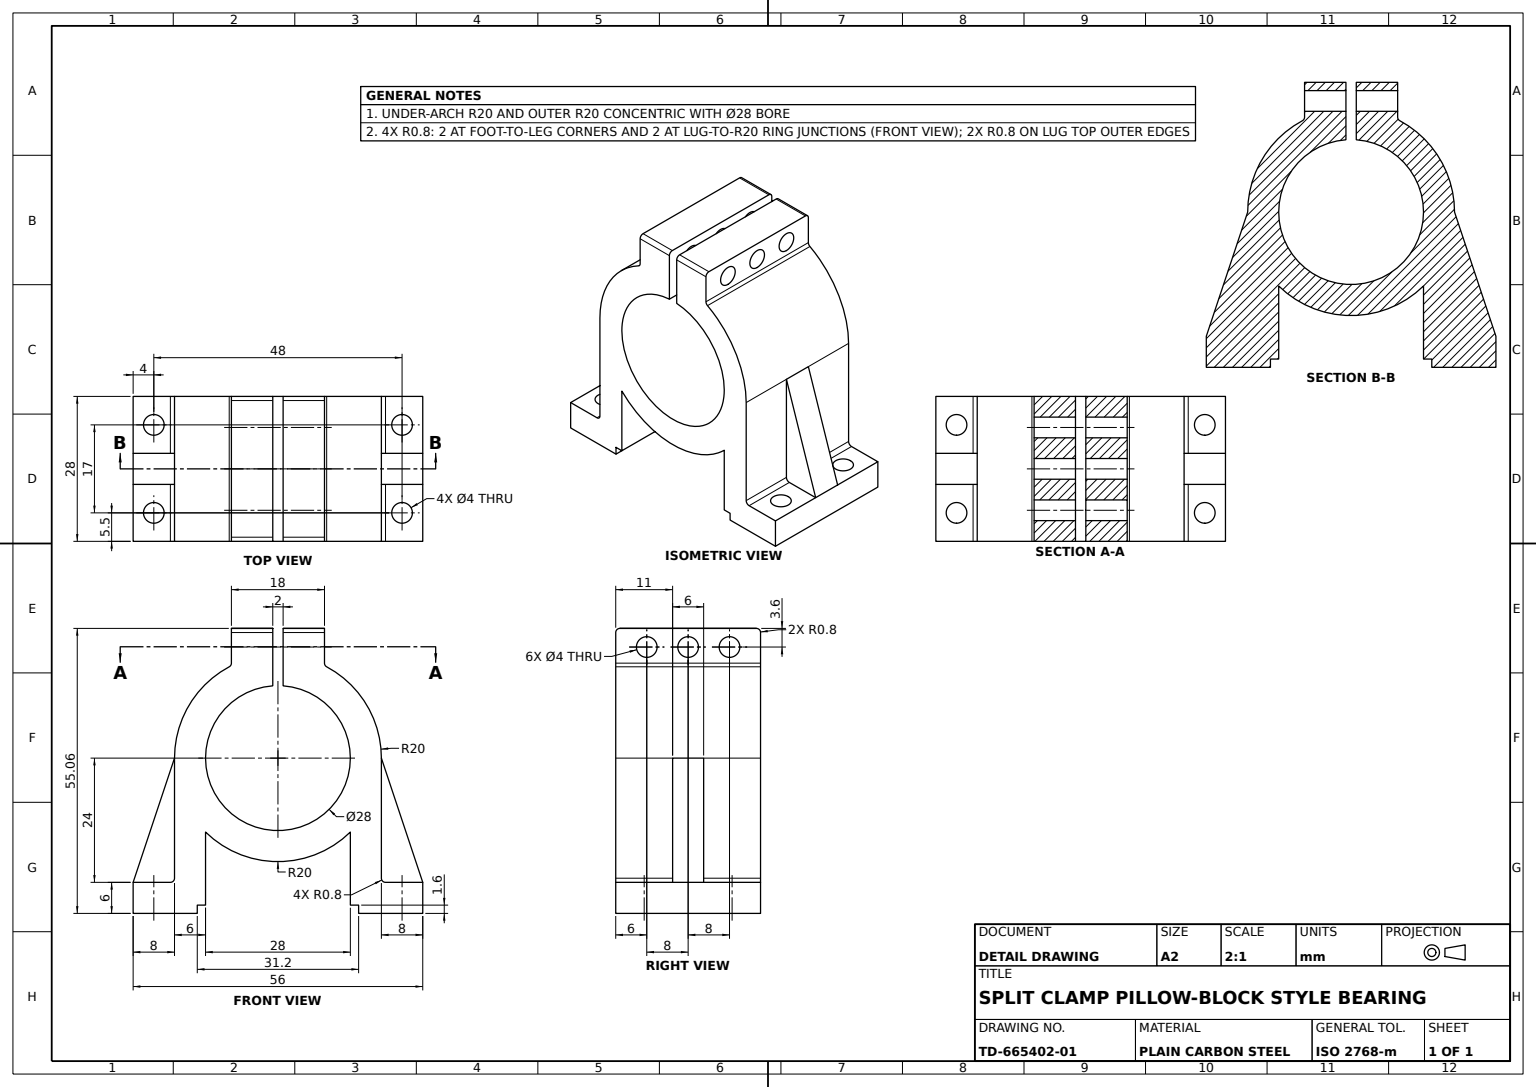
SolidWorks part; units mm, degrees
material "Plain Carbon Steel"
ref_plane "Front Plane" through (0, 0, 0) normal (0, 0, 1) x (1, 0, 0)
ref_plane "Top Plane" through (0, 0, 0) normal (0, 1, 0) x (1, 0, 0)
ref_plane "Right Plane" through (0, 0, 0) normal (1, 0, 0) x (0, 0, -1)
sketch "Omega Profile Sketch" plane through (0, 0, 0) normal (0, 0, 1) x (1, 0, 0)
  line L0 (-20, 0) -> (-20, -24)
  line L1 (-20, -24) -> (-28, -24)
  line L2 (-28, -24) -> (-28, -30)
  line L3 (-28, -30) -> (-15.6, -30)
  line L4 (-14, -28.4) -> (-14, -14.2829)
  line L5 (-14, -28.4) -> (-15.6, -28.4)
  line L6 (-15.6, -28.4) -> (-15.6, -30)
  line L7 (20, 0) -> (20, -24)
  line L8 (20, -24) -> (28, -24)
  line L9 (28, -24) -> (28, -30)
  line L10 (28, -30) -> (15.6, -30)
  line L11 (14, -28.4) -> (14, -14.2829)
  line L12 (14, -28.4) -> (15.6, -28.4)
  line L13 (15.6, -28.4) -> (15.6, -30)
  arc A0 (-14, -14.2829) -> (14, -14.2829) centre (0, 0) ccw
  circle A1 centre (0, 0) radius 14
  arc A2 (20, 0) -> (-20, 0) centre (0, 0) ccw
  dimension "D1" = 40
  dimension "D2" = 28
  dimension "D3" = 8
  dimension "D4" = 24
  dimension "D5" = 6
  dimension "D6" = 1.6
  dimension "D7" = 1.6
  dimension "D8" = 24
  dimension "D9" = 8
  dimension "D10" = 6
  dimension "D11" = 1.6
extrude "Omega Body" add sketch "Omega Profile Sketch" against normal blind 28
ref_plane "Plane1" through (0, 0, -14) normal (0, 0, 1) x (1, 0, 0)
sketch "Support Rib Sketch" plane through (0, 0, -14) normal (0, 0, 1) x (1, 0, 0)
  line L0 (20, 0) -> (28, -24)
rib "Support Rib" sketch "Support Rib Sketch" sketch "Support Rib Sketch" thickness 6 extrusion direction parallel to sketch draft on no parameters "D1"=6
mirror "Support Rib Mirror" about plane through (0, 0, 0) normal (1, 0, 0) of "Support Rib"
sketch "Base Mounting Holes Sketch" plane through (0, -24, 0) normal (0, 1, 0) x (1, 0, 0)
  line L0 (-28, 28) -> (-28, 17) construction
  line L1 (-20, 28) -> (-28, 28) construction
  line L2 (-28, 11) -> (-28, 0) construction
  line L3 (-20, 0) -> (-28, 0) construction
  line L4 (28, 0) -> (20, 0) construction
  line L5 (28, 11) -> (28, 0) construction
  line L6 (28, 28) -> (28, 17) construction
  line L7 (28, 28) -> (20, 28) construction
  circle A0 centre (24, 22.5) radius 2
  circle A1 centre (24, 5.5) radius 2
  circle A2 centre (-24, 5.5) radius 2
  circle A3 centre (-24, 22.5) radius 2
  dimension "D1" = 4
  dimension "D2" = 4
  dimension "D3" = 5.5
  dimension "D4" = 4
  dimension "D5" = 5.5
  dimension "D6" = 5.5
  dimension "D7" = 4
  dimension "D8" = 4
  dimension "D9" = 5.5
extrude "Base Mounting Holes" cut sketch "Base Mounting Holes Sketch" against normal blind 28
sketch "Clamp Lug Sketch" plane through (0, 0, 0) normal (0, 0, 1) x (1, 0, 0)
  line L2 (-9, 17.8606) -> (-9, 25.0606)
  line L3 (-9, 25.0606) -> (9, 25.0606)
  line L4 (9, 17.8606) -> (9, 25.0606)
  arc A1 (20, 0) -> (-20, 0) centre (0, 0) ccw construction
  arc A2 (9, 17.8606) -> (-9, 17.8606) centre (0, 0) ccw
  dimension "D1" = 18
  dimension "D2" = 9
  dimension "D3" = 7.2
extrude "Clamp Lug" add sketch "Clamp Lug Sketch" against normal blind 28
sketch "Split Slot Sketch" plane through (0, 0, 0) normal (0, 0, 1) x (1, 0, 0)
  line L1 (-1, 11.8847) -> (1, 11.8847)
  line L2 (-1, 11.8847) -> (-1, 30.0324)
  line L3 (-1, 30.0324) -> (1, 30.0324)
  line L4 (1, 11.8847) -> (1, 30.0324)
  dimension "D1" = 2
  dimension "D2" = 1
  dimension "D3" = 18.1477
  dimension "D4" = 30.0324
extrude "Split Slot 2mm" cut sketch "Split Slot Sketch" against normal blind 28
sketch "Clamp Screw Holes Sketch" plane through (9, 0, 0) normal (1, 0, 0) x (0, 0, -1)
  line L0 (0, 17.8606) -> (0, 25.0606) construction
  line L1 (28, 25.0606) -> (0, 25.0606) construction
  line L2 (28, 17.8606) -> (0, 17.8606) construction
  circle A0 centre (6, 21.4606) radius 2
  circle A1 centre (14, 21.4606) radius 2
  circle A2 centre (22, 21.4606) radius 2
  dimension "D1" = 4
  dimension "D2" = 14
  dimension "D3" = 3.6
  dimension "D4" = 8
  dimension "D5" = 3.6
  dimension "D6" = 8
  dimension "D7" = 3.6
extrude "Clamp Screw Holes 3xØ3.6" cut sketch "Clamp Screw Holes Sketch" against normal blind 28
fillet "Edge Fillets R0.8" radius 0.8 10 edges at (-9, 17.8606, -14) (5, 25.0606, 0) (5, 25.0606, -28) (-5, 25.0606, -28) (-5, 25.0606, 0) (9, 17.8606, -14) (-20, -24, -5.5) (-20, -24, -22.5) (20, -24, -22.5) (20, -24, -5.5)
